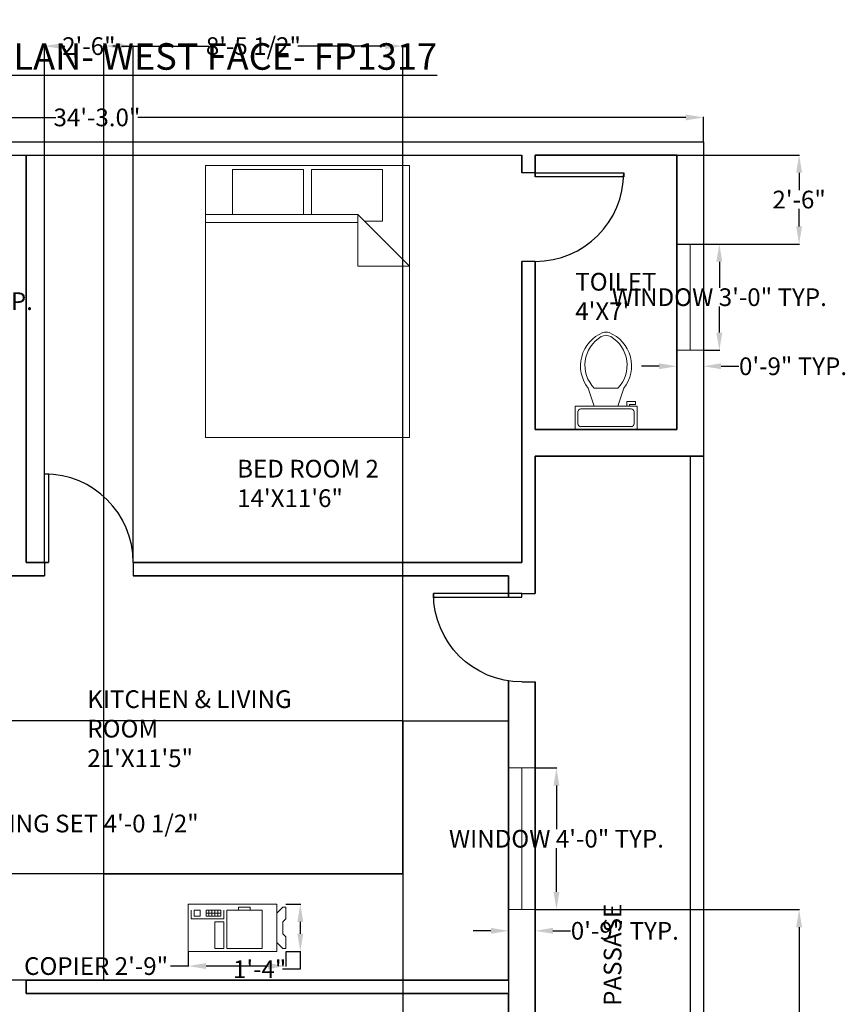
# Model space of a CAD drawing. Units: inches. Extents: x 889 to 1449, y 3224 to 3899.
# Tile 4 of 4: x 1169 to 1449, y 3565 to 3899. Entities that reach past the tile are written whole.
import ezdxf

# ---------------------------------------------------------------- set-up
doc = ezdxf.new("R2010")
doc.units = ezdxf.units.IN
doc.header["$MEASUREMENT"] = 0
for name, color, linetype, lineweight in [('A-ANNO-DIMS', 2, 'Continuous', 18), ('A-ANNO-TEXT', 7, 'Continuous', 25), ('A-AREA-IDEN', 7, 'Continuous', 18), ('A-DOOR', 4, 'Continuous', 25), ('A-EQPM', 9, 'Continuous', 18), ('A-FLOR-CASE', 7, 'Continuous', 25), ('A-FLOR-FIXT', 9, 'Continuous', 18), ('A-FURN', 8, 'Continuous', 18), ('A-GLAZ', 4, 'Continuous', 18), ('A-WALL', 7, 'Continuous', 35), ('C-PROP', 7, 'Continuous', 25)]:
    doc.layers.add(name, color=color, linetype=linetype, lineweight=lineweight)
doc.styles.get("Standard").update_dxf_attribs({"font": 'arial.ttf'})
doc.dimstyles.get("Standard").update_dxf_attribs({"dimtxt": 6, "dimasz": 6, "dimexe": 0.18, "dimexo": 0.0625, "dimgap": 0.09, "dimtad": 0, "dimtih": 1, "dimtoh": 1, "dimdec": 1, "dimzin": 0, "dimdsep": 46, "dimlunit": 3, "dimtxsty": 'Standard', "dimcen": 0.09, "dimadec": 0, "dimazin": 0, "dimtfac": 1, "dimtdec": 1, "dimtofl": 0, "dimtmove": 0, "dimatfit": 3, "dimfxl": 1, "dimtolj": 1, "dimtzin": 0, "dimarcsym": 0})

# ---------------------------------------------------------------- blocks, each defined once
blk = doc.blocks.new('*U2')
for p, q in [((0, 0), (0, -6)), ((40, 0), (40, -6))]:
    blk.add_line(p, q)
blk.add_lwpolyline([(0, 0), (0, 40), (1.75, 40), (1.75, 0)], close=True)
blk.add_arc((0, 0), 40, 0, 90)
blk = doc.blocks.new('Copy Machine')
for p, q in [((0, 0), (0, -16)), ((30, 0), (0, 0)), ((30, -16), (30, 0)), ((-3, -1), (-3, -5)), ((-2, -1), (-3, -1)), ((0, -3), (-2, -1)), ((5, -1), (5, -14)), ((17, -1), (5, -1)), ((17, -14), (17, -1)), ((18, -1), (18, -10)), ((21, -1), (18, -1)), ((21, -10), (21, -1)), ((-3, -5), (-2, -6)), ((-2, -10), (-2, -6)), ((-3, -11), (-2, -10)), ((18, -10), (21, -10)), ((-3, -15), (-3, -11)), ((0, -13), (-2, -15)), ((18, -14), (18, -11)), ((18, -11), (29, -11)), ((24, -12), (19, -12)), ((19, -12), (19, -14)), ((24, -13), (19, -13)), ((20, -12), (20, -14)), ((21, -14), (21, -12)), ((22, -12), (22, -14)), ((23, -14), (23, -12)), ((24, -14), (24, -12)), ((28, -12), (26, -12)), ((26, -12), (26, -14)), ((28, -14), (28, -12)), ((29, -11), (29, -14)), ((-2, -15), (-3, -15)), ((0, -16), (30, -16)), ((5, -14), (17, -14)), ((9, -14), (9, -15)), ((9, -15), (13, -15)), ((13, -15), (13, -14)), ((19, -14), (24, -14)), ((26, -14), (28, -14))]:
    blk.add_line(p, q)
blk = doc.blocks.new('Bed - Queen')
for p, q in [((0, -80.00003), (0, 0)), ((0, 0), (59.99999, 0)), ((59.99999, 0), (59.99999, -80.00003)), ((7.99999, -1.2), (28.79998, -1.2)), ((7.99999, -14.4), (7.99999, -1.2)), ((28.79998, -1.2), (28.79998, -14.4)), ((31.19999, -1.2), (51.99999, -1.2)), ((31.19999, -14.4), (31.19999, -1.2)), ((51.99999, -1.2), (51.99999, -16.4)), ((0, -14.4), (44.8, -14.4)), ((59.99999, -29.6), (44.8, -14.4)), ((44.8, -14.4), (44.8, -29.6)), ((44.8, -16.8), (0, -16.8)), ((51.99999, -16.4), (46.79936, -16.4)), ((44.8, -29.6), (59.99999, -29.6)), ((59.99999, -80.00003), (0, -80.00003))]:
    blk.add_line(p, q)
blk = doc.blocks.new('*U16')
for p, q in [((6, 9.5), (2, 9.5)), ((8, 4), (14, 6)), ((14, 4), (14, -4)), ((8, -4), (14, -6)), ((8, -7), (9.5, -7)), ((8.5, -8), (8, -8)), ((8.5, -10), (8.5, -8)), ((9.5, -10), (8.5, -10)), ((9.5, -7), (9.5, -10))]:
    blk.add_line(p, q)
blk.add_lwpolyline([(8, 10.5), (0, 10.5), (0, -10.5), (8, -10.5)], close=True)
for points in [[(1, 8.5), (1, -8.5)], [(7, -8.5), (7, 8.5)], [(2, -9.5), (6, -9.5)]]:
    blk.add_lwpolyline(points)
for centre, radius, start, end in [((1.87, 8.62), 0.884, 81.8699, 188.1301), ((6.12, 8.62), 0.884, 351.8699, 98.1301), ((21.58, -3.52), 12.17, 22.0284, 128.5307), ((21.82, -4.2), 11.33, 31.053, 133.6321), ((27.88, 0), 4, 335.7318, 24.2682), ((29, 0), 4, 344.8605, 15.1395), ((21.58, 3.52), 12.17, 231.4691, 337.9714), ((21.82, 4.2), 11.33, 226.3677, 328.9468), ((1.87, -8.63), 0.884, 171.8699, 278.1301), ((6.12, -8.63), 0.884, 261.8699, 8.1301)]:
    blk.add_arc(centre, radius, start, end)
blk = doc.blocks.new('*D18')
at = {"layer": 'A-ANNO-DIMS', "color": 0, "lineweight": -2, "transparency": 16777216}
for p, q in [((989.45, 3857.42), (989.45, 3865.8)), ((995.45, 3865.62), (1181.06, 3865.62)), ((1394.45, 3865.62), (1208.83, 3865.62)), ((1400.45, 3857.42), (1400.45, 3865.8))]:
    blk.add_line(p, q, dxfattribs=at)
at = {"layer": 'A-ANNO-DIMS', "color": 0, "transparency": 16777216}
for points in [[(995.45, 3866.62), (995.45, 3864.62), (989.45, 3865.62)], [(1394.45, 3866.62), (1394.45, 3864.62), (1400.45, 3865.62)]]:
    blk.add_solid(points, dxfattribs=at)
at = {"layer": 'Defpoints', "color": 0, "transparency": 16777216}
for p in [(1400.45, 3865.62), (989.45, 3857.35), (1400.45, 3857.35)]:
    blk.add_point(p, dxfattribs=at)
at = {"layer": 'A-ANNO-DIMS', "color": 0, "transparency": 16777216, "insert": (1194.95, 3865.62), "char_height": 6, "attachment_point": 5}
blk.add_mtext('\\A1;34\'-3.0"', dxfattribs=at)
blk = doc.blocks.new('WIN-48IN')
blk.add_line((4.5, 48), (4.5, 0))
blk.add_lwpolyline([(9, 48), (9, 0), (0, 0), (0, 48)], close=True)
blk = doc.blocks.new('WIN-36IN')
blk.add_line((4.5, 36), (4.5, 0))
blk.add_lwpolyline([(9, 36), (9, 0), (0, 0), (0, 36)], close=True)
blk = doc.blocks.new('*D26')
at = {"layer": 'A-ANNO-DIMS', "color": 0, "lineweight": -2, "transparency": 16777216}
for p, q in [((1343.51, 3645.24), (1350.83, 3645.24)), ((1350.65, 3639.24), (1350.65, 3624.43)), ((1350.65, 3603.24), (1350.65, 3618.04)), ((1343.51, 3597.24), (1350.83, 3597.24))]:
    blk.add_line(p, q, dxfattribs=at)
at = {"layer": 'A-ANNO-DIMS', "color": 0, "transparency": 16777216}
for points in [[(1349.65, 3639.24), (1351.65, 3639.24), (1350.65, 3645.24)], [(1349.65, 3603.24), (1351.65, 3603.24), (1350.65, 3597.24)]]:
    blk.add_solid(points, dxfattribs=at)
at = {"layer": 'Defpoints', "color": 0, "transparency": 16777216}
for p in [(1343.45, 3645.24), (1350.65, 3645.24), (1343.45, 3597.24)]:
    blk.add_point(p, dxfattribs=at)
at = {"layer": 'A-ANNO-DIMS', "color": 0, "transparency": 16777216, "insert": (1350.65, 3621.24), "char_height": 6, "attachment_point": 5}
blk.add_mtext('\\A1;WINDOW 4\'-0" TYP.', dxfattribs=at)
blk = doc.blocks.new('*D27')
at = {"layer": 'A-ANNO-DIMS', "color": 0, "lineweight": -2, "transparency": 16777216}
for p, q in [((1334.45, 3597.18), (1334.45, 3589.86)), ((1343.45, 3597.18), (1343.45, 3589.86)), ((1328.45, 3590.04), (1322.45, 3590.04)), ((1349.45, 3590.04), (1355.45, 3590.04))]:
    blk.add_line(p, q, dxfattribs=at)
at = {"layer": 'A-ANNO-DIMS', "color": 0, "transparency": 16777216}
for points in [[(1328.45, 3591.04), (1328.45, 3589.04), (1334.45, 3590.04)], [(1349.45, 3591.04), (1349.45, 3589.04), (1343.45, 3590.04)]]:
    blk.add_solid(points, dxfattribs=at)
at = {"layer": 'Defpoints', "color": 0, "transparency": 16777216}
for p in [(1334.45, 3597.24), (1343.45, 3597.24), (1343.45, 3590.04)]:
    blk.add_point(p, dxfattribs=at)
at = {"layer": 'A-ANNO-DIMS', "color": 0, "transparency": 16777216, "insert": (1373.82, 3590.04), "char_height": 6, "attachment_point": 5}
blk.add_mtext('\\A1;0\'-9" TYP.', dxfattribs=at)
blk = doc.blocks.new('*D28')
at = {"layer": 'A-ANNO-DIMS', "color": 0, "lineweight": -2, "transparency": 16777216}
for p, q in [((1400.51, 3822.72), (1406.03, 3822.72)), ((1405.85, 3816.72), (1405.85, 3807.92)), ((1405.85, 3792.72), (1405.85, 3801.52)), ((1400.51, 3786.72), (1406.03, 3786.72))]:
    blk.add_line(p, q, dxfattribs=at)
at = {"layer": 'A-ANNO-DIMS', "color": 0, "transparency": 16777216}
for points in [[(1404.85, 3816.72), (1406.85, 3816.72), (1405.85, 3822.72)], [(1404.85, 3792.72), (1406.85, 3792.72), (1405.85, 3786.72)]]:
    blk.add_solid(points, dxfattribs=at)
at = {"layer": 'Defpoints', "color": 0, "transparency": 16777216}
for p in [(1400.45, 3822.72), (1405.85, 3822.72), (1400.45, 3786.72)]:
    blk.add_point(p, dxfattribs=at)
at = {"layer": 'A-ANNO-DIMS', "color": 0, "transparency": 16777216, "insert": (1405.85, 3804.72), "char_height": 6, "attachment_point": 5}
blk.add_mtext('\\A1;WINDOW 3\'-0" TYP.', dxfattribs=at)
blk = doc.blocks.new('*D29')
at = {"layer": 'A-ANNO-DIMS', "color": 0, "lineweight": -2, "transparency": 16777216}
for p, q in [((1391.45, 3786.66), (1391.45, 3781.14)), ((1400.45, 3786.66), (1400.45, 3781.14)), ((1385.45, 3781.32), (1379.45, 3781.32)), ((1406.45, 3781.32), (1412.45, 3781.32))]:
    blk.add_line(p, q, dxfattribs=at)
at = {"layer": 'A-ANNO-DIMS', "color": 0, "transparency": 16777216}
for points in [[(1385.45, 3782.32), (1385.45, 3780.32), (1391.45, 3781.32)], [(1406.45, 3782.32), (1406.45, 3780.32), (1400.45, 3781.32)]]:
    blk.add_solid(points, dxfattribs=at)
at = {"layer": 'Defpoints', "color": 0, "transparency": 16777216}
for p in [(1391.45, 3786.72), (1400.45, 3786.72), (1400.45, 3781.32)]:
    blk.add_point(p, dxfattribs=at)
at = {"layer": 'A-ANNO-DIMS', "color": 0, "transparency": 16777216, "insert": (1430.82, 3781.32), "char_height": 6, "attachment_point": 5}
blk.add_mtext('\\A1;0\'-9" TYP.', dxfattribs=at)
blk = doc.blocks.new('*D30')
at = {"layer": 'A-ANNO-DIMS', "color": 0, "lineweight": -2, "transparency": 16777216}
for p, q in [((1117.62, 3849.48), (1131.58, 3849.48)), ((1131.4, 3843.48), (1131.4, 3806.74)), ((1131.4, 3763.24), (1131.4, 3799.99)), ((1117.62, 3757.24), (1131.58, 3757.24))]:
    blk.add_line(p, q, dxfattribs=at)
at = {"layer": 'A-ANNO-DIMS', "color": 0, "transparency": 16777216}
for points in [[(1130.4, 3843.48), (1132.4, 3843.48), (1131.4, 3849.48)], [(1130.4, 3763.24), (1132.4, 3763.24), (1131.4, 3757.24)]]:
    blk.add_solid(points, dxfattribs=at)
at = {"layer": 'Defpoints', "color": 0, "transparency": 16777216}
for p in [(1117.56, 3849.48), (1131.4, 3849.48), (1117.56, 3757.24)]:
    blk.add_point(p, dxfattribs=at)
at = {"layer": 'A-ANNO-DIMS', "color": 0, "transparency": 16777216, "insert": (1131.4, 3803.36), "char_height": 6, "attachment_point": 5}
blk.add_mtext('\\A1;QUEEN BED 7\'-8" TYP.', dxfattribs=at)
blk = doc.blocks.new('*D36')
at = {"layer": 'A-ANNO-DIMS', "color": 0, "lineweight": -2, "transparency": 16777216}
for p, q in [((1095.64, 3633.61), (1095.64, 3626.21)), ((1144.17, 3633.61), (1144.17, 3626.21)), ((1101.64, 3626.39), (1138.17, 3626.39)), ((1144.17, 3626.39), (1150.17, 3626.39))]:
    blk.add_line(p, q, dxfattribs=at)
at = {"layer": 'A-ANNO-DIMS', "color": 0, "transparency": 16777216}
for points in [[(1101.64, 3627.39), (1101.64, 3625.39), (1095.64, 3626.39)], [(1138.17, 3627.39), (1138.17, 3625.39), (1144.17, 3626.39)]]:
    blk.add_solid(points, dxfattribs=at)
at = {"layer": 'Defpoints', "color": 0, "transparency": 16777216}
for p in [(1095.64, 3633.67), (1144.17, 3633.67), (1144.17, 3626.39)]:
    blk.add_point(p, dxfattribs=at)
at = {"layer": 'A-ANNO-DIMS', "color": 0, "transparency": 16777216, "insert": (1190.23, 3626.39), "char_height": 6, "attachment_point": 5}
blk.add_mtext('\\A1;DINING SET 4\'-0 1/2"', dxfattribs=at)
blk = doc.blocks.new('*D38')
at = {"layer": 'A-ANNO-DIMS', "color": 0, "lineweight": -2, "transparency": 16777216}
for p, q in [((1225.91, 3582.98), (1225.91, 3577.92)), ((1258.91, 3582.98), (1258.91, 3577.92)), ((1225.91, 3578.1), (1219.91, 3578.1)), ((1252.91, 3578.1), (1231.91, 3578.1))]:
    blk.add_line(p, q, dxfattribs=at)
at = {"layer": 'A-ANNO-DIMS', "color": 0, "transparency": 16777216}
for points in [[(1231.91, 3579.1), (1231.91, 3577.1), (1225.91, 3578.1)], [(1252.91, 3579.1), (1252.91, 3577.1), (1258.91, 3578.1)]]:
    blk.add_solid(points, dxfattribs=at)
at = {"layer": 'Defpoints', "color": 0, "transparency": 16777216}
for p in [(1225.91, 3583.05), (1258.91, 3583.05), (1225.91, 3578.1)]:
    blk.add_point(p, dxfattribs=at)
at = {"layer": 'A-ANNO-DIMS', "color": 0, "transparency": 16777216, "insert": (1194.65, 3578.1), "char_height": 6, "attachment_point": 5}
blk.add_mtext('\\A1;COPIER 2\'-9"', dxfattribs=at)
blk = doc.blocks.new('*D39')
at = {"layer": 'A-ANNO-DIMS', "color": 0, "lineweight": -2, "transparency": 16777216}
for p, q in [((1258.97, 3599.05), (1264.04, 3599.05)), ((1263.86, 3593.05), (1263.86, 3589.05)), ((1258.97, 3583.05), (1264.04, 3583.05)), ((1263.86, 3583.05), (1263.86, 3577.05)), ((1263.86, 3577.05), (1257.86, 3577.05))]:
    blk.add_line(p, q, dxfattribs=at)
at = {"layer": 'A-ANNO-DIMS', "color": 0, "transparency": 16777216}
for points in [[(1262.86, 3593.05), (1264.86, 3593.05), (1263.86, 3599.05)], [(1262.86, 3589.05), (1264.86, 3589.05), (1263.86, 3583.05)]]:
    blk.add_solid(points, dxfattribs=at)
at = {"layer": 'Defpoints', "color": 0, "transparency": 16777216}
for p in [(1258.91, 3599.05), (1258.91, 3583.05), (1263.86, 3583.05)]:
    blk.add_point(p, dxfattribs=at)
at = {"layer": 'A-ANNO-DIMS', "color": 0, "transparency": 16777216, "insert": (1250.08, 3577.05), "char_height": 6, "attachment_point": 5}
blk.add_mtext('\\A1;1\'-4"', dxfattribs=at)
blk = doc.blocks.new('*D49')
at = {"layer": 'A-ANNO-DIMS', "color": 0, "lineweight": -2, "transparency": 16777216}
for p, q in [((1177.21, 3714.92), (1177.21, 3889.96)), ((1183.21, 3889.78), (1184.09, 3889.78)), ((1201.21, 3889.78), (1200.32, 3889.78)), ((1207.21, 3714.92), (1207.21, 3889.96))]:
    blk.add_line(p, q, dxfattribs=at)
at = {"layer": 'A-ANNO-DIMS', "color": 0, "transparency": 16777216}
for points in [[(1183.21, 3890.78), (1183.21, 3888.78), (1177.21, 3889.78)], [(1201.21, 3890.78), (1201.21, 3888.78), (1207.21, 3889.78)]]:
    blk.add_solid(points, dxfattribs=at)
at = {"layer": 'Defpoints', "color": 0, "transparency": 16777216}
for p in [(1207.21, 3889.78), (1177.21, 3714.85), (1207.21, 3714.85)]:
    blk.add_point(p, dxfattribs=at)
at = {"layer": 'A-ANNO-DIMS', "color": 0, "transparency": 16777216, "insert": (1192.21, 3889.78), "char_height": 6, "attachment_point": 5}
blk.add_mtext('\\A1;2\'-6"', dxfattribs=at)
blk = doc.blocks.new('*D51')
at = {"layer": 'A-ANNO-DIMS', "color": 0, "lineweight": -2, "transparency": 16777216}
for p, q in [((1343.51, 3597.24), (1433.06, 3597.24)), ((1432.88, 3591.24), (1432.88, 3557.7)), ((1432.88, 3517.78), (1432.88, 3551.32)), ((1343.51, 3511.78), (1433.06, 3511.78))]:
    blk.add_line(p, q, dxfattribs=at)
at = {"layer": 'A-ANNO-DIMS', "color": 0, "transparency": 16777216}
for points in [[(1431.88, 3591.24), (1433.88, 3591.24), (1432.88, 3597.24)], [(1431.88, 3517.78), (1433.88, 3517.78), (1432.88, 3511.78)]]:
    blk.add_solid(points, dxfattribs=at)
at = {"layer": 'Defpoints', "color": 0, "transparency": 16777216}
for p in [(1343.45, 3597.24), (1432.88, 3597.24), (1343.45, 3511.78)]:
    blk.add_point(p, dxfattribs=at)
at = {"layer": 'A-ANNO-DIMS', "color": 0, "transparency": 16777216, "insert": (1432.88, 3554.51), "char_height": 6, "attachment_point": 5}
blk.add_mtext('\\A1;7\'-1 1/2"', dxfattribs=at)
blk = doc.blocks.new('*D55')
at = {"layer": 'A-ANNO-DIMS', "color": 0, "lineweight": -2, "transparency": 16777216}
for p, q in [((1391.51, 3852.85), (1433.06, 3852.85)), ((1432.88, 3846.85), (1432.88, 3840.94)), ((1432.88, 3828.72), (1432.88, 3834.63)), ((1391.51, 3822.72), (1433.06, 3822.72))]:
    blk.add_line(p, q, dxfattribs=at)
at = {"layer": 'A-ANNO-DIMS', "color": 0, "transparency": 16777216}
for points in [[(1431.88, 3846.85), (1433.88, 3846.85), (1432.88, 3852.85)], [(1431.88, 3828.72), (1433.88, 3828.72), (1432.88, 3822.72)]]:
    blk.add_solid(points, dxfattribs=at)
at = {"layer": 'Defpoints', "color": 0, "transparency": 16777216}
for p in [(1391.45, 3852.85), (1432.88, 3852.85), (1391.45, 3822.72)]:
    blk.add_point(p, dxfattribs=at)
at = {"layer": 'A-ANNO-DIMS', "color": 0, "transparency": 16777216, "insert": (1432.88, 3837.79), "char_height": 6, "attachment_point": 5}
blk.add_mtext('\\A1;2\'-6"', dxfattribs=at)
blk = doc.blocks.new('*D58')
at = {"layer": 'A-ANNO-DIMS', "color": 0, "lineweight": -2, "transparency": 16777216}
for p, q in [((1197.23, 3609.35), (907.11, 3609.35)), ((907.29, 3603.35), (907.29, 3594.51)), ((907.29, 3579.35), (907.29, 3588.2)), ((1197.23, 3573.35), (907.11, 3573.35))]:
    blk.add_line(p, q, dxfattribs=at)
at = {"layer": 'A-ANNO-DIMS', "color": 0, "transparency": 16777216}
for points in [[(906.29, 3603.35), (908.29, 3603.35), (907.29, 3609.35)], [(906.29, 3579.35), (908.29, 3579.35), (907.29, 3573.35)]]:
    blk.add_solid(points, dxfattribs=at)
at = {"layer": 'Defpoints', "color": 0, "transparency": 16777216}
for p in [(907.29, 3609.35), (1197.3, 3609.35), (1197.3, 3573.35)]:
    blk.add_point(p, dxfattribs=at)
at = {"layer": 'A-ANNO-DIMS', "color": 0, "transparency": 16777216, "insert": (907.29, 3591.35), "char_height": 6, "attachment_point": 5}
blk.add_mtext('\\A1;3\'-0"', dxfattribs=at)
blk = doc.blocks.new('*D59')
at = {"layer": 'A-ANNO-DIMS', "color": 0, "lineweight": -2, "transparency": 16777216}
for p, q in [((1197.3, 3609.42), (1197.3, 3889.96)), ((1203.3, 3889.78), (1232.9, 3889.78)), ((1292.62, 3889.78), (1263.02, 3889.78)), ((1298.62, 3609.42), (1298.62, 3889.96))]:
    blk.add_line(p, q, dxfattribs=at)
at = {"layer": 'A-ANNO-DIMS', "color": 0, "transparency": 16777216}
for points in [[(1203.3, 3890.78), (1203.3, 3888.78), (1197.3, 3889.78)], [(1292.62, 3890.78), (1292.62, 3888.78), (1298.62, 3889.78)]]:
    blk.add_solid(points, dxfattribs=at)
at = {"layer": 'Defpoints', "color": 0, "transparency": 16777216}
for p in [(1298.62, 3889.78), (1197.3, 3609.35), (1298.62, 3609.35)]:
    blk.add_point(p, dxfattribs=at)
at = {"layer": 'A-ANNO-DIMS', "color": 0, "transparency": 16777216, "insert": (1247.96, 3889.78), "char_height": 6, "attachment_point": 5}
blk.add_mtext('\\A1;8\'-5 1/2"', dxfattribs=at)
blk = doc.blocks.new('*D60')
at = {"layer": 'A-ANNO-DIMS', "color": 0, "lineweight": -2, "transparency": 16777216}
for p, q in [((1298.62, 3661.08), (1298.62, 3232.74)), ((1334.45, 3661.08), (1334.45, 3232.74)), ((1304.62, 3232.92), (1308.47, 3232.92)), ((1328.45, 3232.92), (1324.6, 3232.92))]:
    blk.add_line(p, q, dxfattribs=at)
at = {"layer": 'A-ANNO-DIMS', "color": 0, "transparency": 16777216}
for points in [[(1304.62, 3233.92), (1304.62, 3231.92), (1298.62, 3232.92)], [(1328.45, 3233.92), (1328.45, 3231.92), (1334.45, 3232.92)]]:
    blk.add_solid(points, dxfattribs=at)
at = {"layer": 'Defpoints', "color": 0, "transparency": 16777216}
for p in [(1298.62, 3661.14), (1334.45, 3661.14), (1334.45, 3232.92)]:
    blk.add_point(p, dxfattribs=at)
at = {"layer": 'A-ANNO-DIMS', "color": 0, "transparency": 16777216, "insert": (1316.53, 3232.92), "char_height": 6, "attachment_point": 5}
blk.add_mtext('\\A1;3\'-0"', dxfattribs=at)
blk = doc.blocks.new('*D61')
at = {"layer": 'A-ANNO-DIMS', "color": 0, "lineweight": -2, "transparency": 16777216}
for p, q in [((1298.56, 3661.14), (907.11, 3661.14)), ((907.29, 3655.14), (907.29, 3638.34)), ((907.29, 3615.35), (907.29, 3632.16)), ((1298.56, 3609.35), (907.11, 3609.35))]:
    blk.add_line(p, q, dxfattribs=at)
at = {"layer": 'A-ANNO-DIMS', "color": 0, "transparency": 16777216}
for points in [[(906.29, 3655.14), (908.29, 3655.14), (907.29, 3661.14)], [(906.29, 3615.35), (908.29, 3615.35), (907.29, 3609.35)]]:
    blk.add_solid(points, dxfattribs=at)
at = {"layer": 'Defpoints', "color": 0, "transparency": 16777216}
for p in [(907.29, 3661.14), (1298.62, 3661.14), (1298.62, 3609.35)]:
    blk.add_point(p, dxfattribs=at)
at = {"layer": 'A-ANNO-DIMS', "color": 0, "transparency": 16777216, "insert": (907.29, 3635.25), "char_height": 6, "attachment_point": 5}
blk.add_mtext('\\A1;4\'-4"', dxfattribs=at)

msp = doc.modelspace()

# ---------------------------------------------------------------- linework, layer by layer
at = {"layer": 'A-FLOR-CASE'}
for p, q in [((1298.62, 3609.35), (1298.62, 3661.14)), ((1298.62, 3661.14), (1334.45, 3661.14)), ((1197.3, 3573.35), (1197.3, 3609.35)), ((1197.3, 3609.35), (1298.62, 3609.35))]:
    msp.add_line(p, q, dxfattribs=at)
at = {"layer": 'A-WALL'}
for p, q in [((1170.95, 3852.85), (1170.95, 3714.85)), ((1338.95, 3852.85), (1338.95, 3846.85)), ((1343.45, 3852.85), (1343.45, 3845.54)), ((1343.45, 3852.85), (1391.45, 3852.85)), ((1391.45, 3852.85), (1391.45, 3759.85)), ((1338.95, 3816.85), (1338.95, 3714.85)), ((1343.45, 3816.85), (1343.45, 3759.85)), ((1343.45, 3759.85), (1391.45, 3759.85)), ((1343.45, 3750.85), (1400.45, 3750.85)), ((1343.45, 3750.85), (1343.45, 3704.35)), ((1170.95, 3714.85), (1178.52, 3714.85)), ((1207.21, 3714.85), (1338.95, 3714.85)), ((1160.18, 3710.35), (1177.21, 3710.35)), ((1207.21, 3710.35), (1334.45, 3710.35)), ((1334.45, 3710.35), (1334.45, 3703.04)), ((1334.45, 3674.69), (1334.45, 3573.35)), ((1343.45, 3674.35), (1343.45, 3403.85)), ((1170.95, 3573.35), (1334.45, 3573.35)), ((1170.95, 3573.35), (1170.95, 3568.85)), ((1170.95, 3568.85), (1334.45, 3568.85)), ((1334.45, 3568.85), (1334.45, 3412.85))]:
    msp.add_line(p, q, dxfattribs=at)
at = {"layer": 'C-PROP'}
for p, q in [((947.95, 3857.35), (1400.45, 3857.35)), ((1400.45, 3857.35), (1400.45, 3265.35)), ((952.45, 3852.85), (1338.95, 3852.85)), ((1395.95, 3750.85), (1395.95, 3269.85))]:
    msp.add_line(p, q, dxfattribs=at)

# ---------------------------------------------------------------- block references
at = {"layer": 'A-DOOR', "yscale": 0.75, "zscale": 0.75}
for p, xscale, rotation in [((1343.45, 3846.85), 0.75, 270), ((1338.95, 3704.35), -0.75, 90)]:
    msp.add_blockref('*U2', p, dxfattribs=dict(at, xscale=xscale, rotation=rotation))
at = {"layer": 'A-DOOR', "xscale": 0.75, "yscale": 0.75, "zscale": 0.75}
msp.add_blockref('*U2', (1177.21, 3714.85), dxfattribs=at)
at = {"layer": 'A-EQPM', "rotation": 180}
msp.add_blockref('Copy Machine', (1255.91, 3583.05), dxfattribs=at)
at = {"layer": 'A-FLOR-FIXT', "rotation": 90}
msp.add_blockref('*U16', (1367.45, 3759.85), dxfattribs=at)
at = {"layer": 'A-FURN', "xscale": 1.153040595648429, "yscale": 1.153040595648429, "zscale": 1.153040595648429}
msp.add_blockref('Bed - Queen', (1231.71, 3849.37), dxfattribs=at)
at = {"layer": 'A-GLAZ'}
for name, p in [('WIN-36IN', (1391.45, 3786.72)), ('WIN-48IN', (1334.45, 3597.24))]:
    msp.add_blockref(name, p, dxfattribs=at)

# ---------------------------------------------------------------- texts
at = {"layer": 'A-ANNO-TEXT', "insert": (1003.26, 3890.77), "char_height": 9, "attachment_point": 1}
msp.add_mtext_dynamic_manual_height_columns('{\\fArial|b1|i0|c0|p34;\\L38X50 (1900 SQ FT) HOUSE PLAN- WEST FACE- FP1317}', width=396.8668, gutter_width=1, heights=[0], dxfattribs=at)
at = {"layer": 'A-AREA-IDEN', "char_height": 6, "attachment_point": 1}
for s, insert in [("TOILET\\P4'X7'", (1357.02, 3812.95)), ('BED ROOM 2\\P14\'X11\'6"', (1242.45, 3749.62)), ('KITCHEN & LIVING ROOM\\P21\'X11\'5"', (1191.67, 3671.53))]:
    msp.add_mtext_dynamic_manual_height_columns(s, width=93.4406, gutter_width=1, heights=[0], dxfattribs=dict(at, insert=insert))
at = {"layer": 'A-AREA-IDEN', "insert": (1366.68, 3564.62), "char_height": 6, "attachment_point": 1, "rotation": 90}
msp.add_mtext_dynamic_manual_height_columns('PASSASE', width=93.4406, gutter_width=1, heights=[0], dxfattribs=at)

# ---------------------------------------------------------------- dimensions: what is measured, and where the dimension line sits
at = {"layer": 'A-ANNO-DIMS'}
for base, p1, p2, override, picture, middle in [((1298.62, 3889.78), (1197.3, 3609.35), (1298.62, 3609.35), {"dimdec": 1, "dimlfac": 1, "dimrnd": 0, "dimzin": 1, "dimdsep": 46, "dimlunit": 4, "dimfrac": 2}, '*D59', (1247.96, 3889.78)), ((1207.21, 3889.78), (1177.21, 3714.85), (1207.21, 3714.85), {"dimdec": 1, "dimlfac": 1, "dimrnd": 0, "dimzin": 1, "dimdsep": 46, "dimlunit": 4, "dimfrac": 2}, '*D49', (1192.21, 3889.78)), ((1400.45, 3865.62), (989.45, 3857.35), (1400.45, 3857.35), {"dimclrd": 0, "dimclre": 0, "dimclrt": 0, "dimtmove": 1}, '*D18', (1194.95, 3865.62)), ((1334.45, 3232.92), (1298.62, 3661.14), (1334.45, 3661.14), {"dimdec": 1, "dimlfac": 1, "dimrnd": 0, "dimzin": 1, "dimdsep": 46, "dimlunit": 4, "dimfrac": 2}, '*D60', (1316.53, 3232.92))]:
    dim = msp.add_linear_dim(base=base, p1=p1, p2=p2, dimstyle='Standard', override=override, dxfattribs=at)
    dim.commit()
    dim.dimension.update_dxf_attribs({"geometry": picture, "text_midpoint": middle})
for base, p1, p2, angle, picture, middle in [((1432.88, 3852.85), (1391.45, 3822.72), (1391.45, 3852.85), 90, '*D55', (1432.88, 3837.79)), ((907.29, 3661.14), (1298.62, 3609.35), (1298.62, 3661.14), 90, '*D61', (907.29, 3635.25)), ((907.29, 3609.35), (1197.3, 3573.35), (1197.3, 3609.35), 90, '*D58', (907.29, 3591.35)), ((1263.86, 3583.05), (1258.91, 3599.05), (1258.91, 3583.05), 270, '*D39', (1250.08, 3577.05)), ((1432.88, 3597.24), (1343.45, 3511.78), (1343.45, 3597.24), 90, '*D51', (1432.88, 3554.51))]:
    dim = msp.add_linear_dim(base=base, p1=p1, p2=p2, angle=angle, dimstyle='Standard', override={"dimdec": 1, "dimlfac": 1, "dimrnd": 0, "dimzin": 1, "dimdsep": 46, "dimlunit": 4, "dimfrac": 2}, dxfattribs=at)
    dim.commit()
    dim.dimension.update_dxf_attribs({"geometry": picture, "text_midpoint": middle})
for base, p1, p2, angle, text, picture, middle in [((1131.4, 3849.48), (1117.56, 3757.24), (1117.56, 3849.48), 90, 'QUEEN BED <> TYP.', '*D30', (1131.4, 3803.36)), ((1405.85, 3822.72), (1400.45, 3786.72), (1400.45, 3822.72), 90, 'WINDOW <> TYP.', '*D28', (1405.85, 3804.72)), ((1350.65, 3645.24), (1343.45, 3597.24), (1343.45, 3645.24), 90, 'WINDOW <> TYP.', '*D26', (1350.65, 3621.24)), ((1225.91, 3578.1), (1258.91, 3583.05), (1225.91, 3583.05), 180, 'COPIER <>', '*D38', (1194.65, 3578.1))]:
    dim = msp.add_linear_dim(base=base, p1=p1, p2=p2, angle=angle, text=text, dimstyle='Standard', override={"dimdec": 1, "dimlfac": 1, "dimrnd": 0, "dimzin": 1, "dimdsep": 46, "dimlunit": 4, "dimfrac": 2}, dxfattribs=at)
    dim.commit()
    dim.dimension.update_dxf_attribs({"geometry": picture, "text_midpoint": middle})
for base, p1, p2, text, picture, middle in [((1400.45, 3781.32), (1391.45, 3786.72), (1400.45, 3786.72), '<> TYP.', '*D29', (1430.82, 3781.32)), ((1144.17, 3626.39), (1095.64, 3633.67), (1144.17, 3633.67), 'DINING SET <>', '*D36', (1190.23, 3626.39)), ((1343.45, 3590.04), (1334.45, 3597.24), (1343.45, 3597.24), '<> TYP.', '*D27', (1373.82, 3590.04))]:
    dim = msp.add_linear_dim(base=base, p1=p1, p2=p2, text=text, dimstyle='Standard', override={"dimdec": 1, "dimlfac": 1, "dimrnd": 0, "dimzin": 1, "dimdsep": 46, "dimlunit": 4, "dimfrac": 2}, dxfattribs=at)
    dim.commit()
    dim.dimension.update_dxf_attribs({"geometry": picture, "text_midpoint": middle})

doc.saveas('drawing.dxf')
